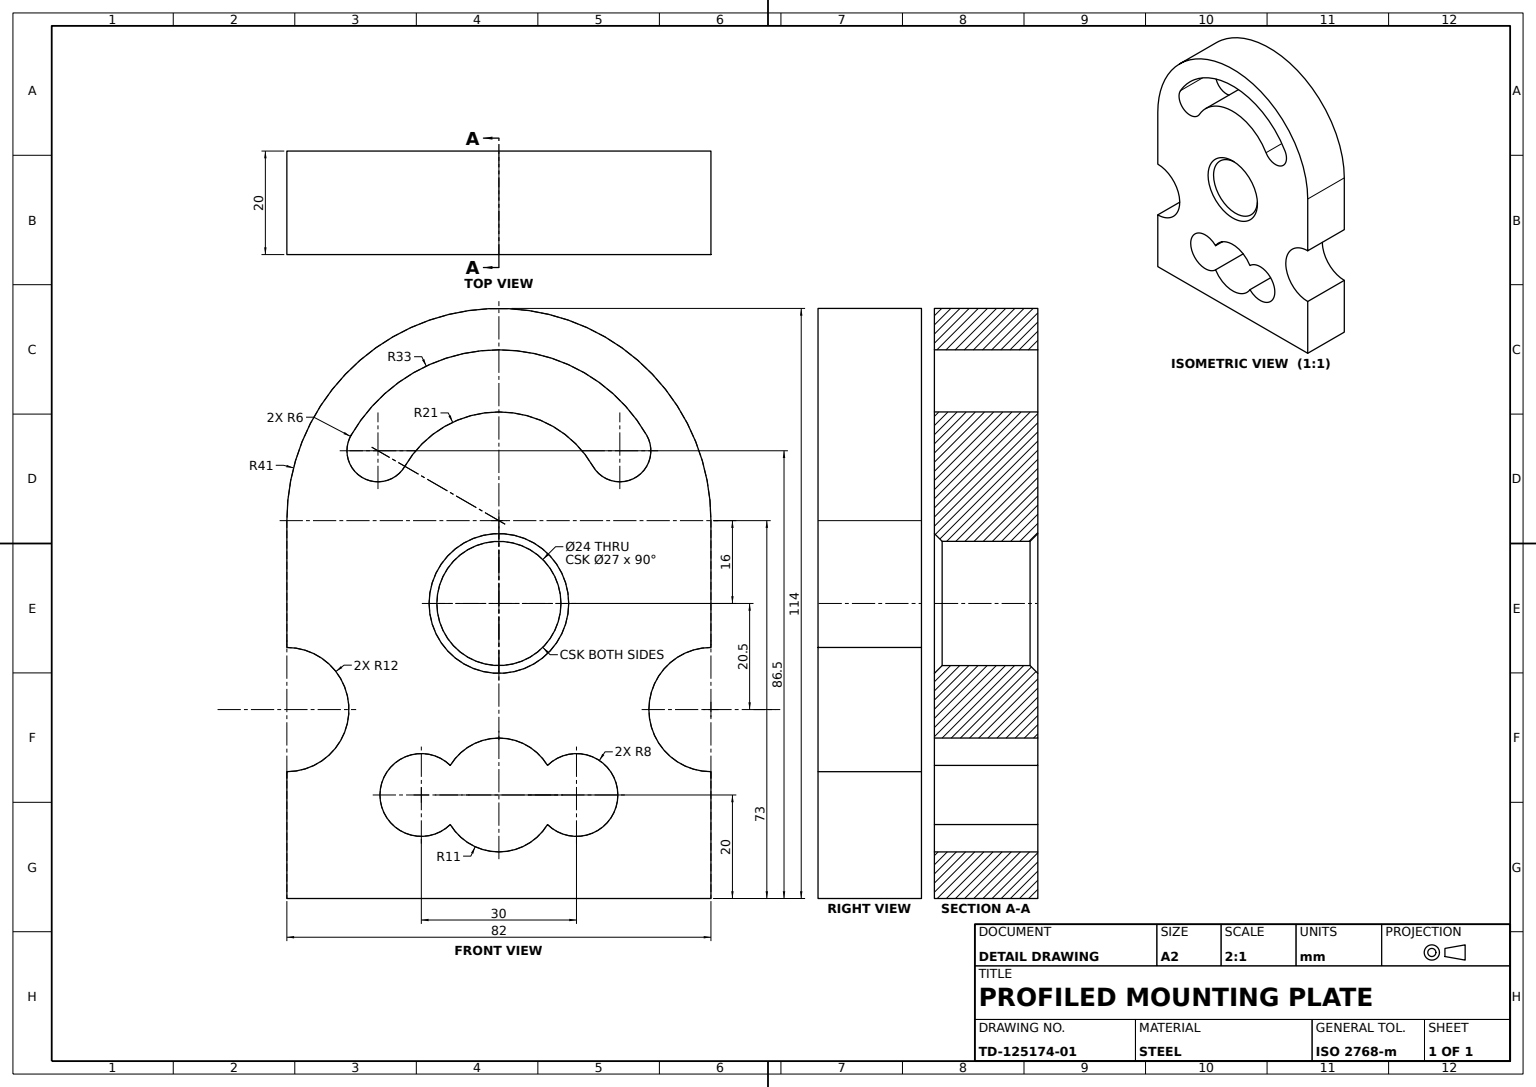
from build123d import *

# Parameters (mm, degrees)
PLATE_PROFILE_SKETCH_R      = 12
PROFILED_PLATE_20MM_DEPTH   = 20
BORE_CHAMFER_1_5X45DEG_SIZE = 1.5


with BuildPart() as part:
    # Plate Profile Sketch → Profiled Plate 20mm (new body)
    with BuildSketch(Plane(origin=(0, 0, 0), x_dir=(0, 0, -1), z_dir=(1, 0, 0))):
        with BuildLine():
            Line((41, 73), (41, 48.5))
            ThreePointArc((41, 48.5), (29, 36.5), (41, 24.5))
            Line((41, 24.5), (41, 0))
            Line((41, 0), (0, 0))
            Line((0, 0), (-41, 0))
            Line((-41, 0), (-41, 24.5))
            ThreePointArc((-41, 24.5), (-29, 36.5), (-41, 48.5))
            Line((-41, 48.5), (-41, 73))
            ThreePointArc((-41, 73), (0, 114), (41, 73))
        make_face()
        with Locations((0, 57)):
            Circle(PLATE_PROFILE_SKETCH_R, mode=Mode.SUBTRACT)
        with BuildLine():
            ThreePointArc((9.4, 25.713142743), (0, 31), (-9.4, 25.713142743))
            ThreePointArc((-9.4, 25.713142743), (-23, 20), (-9.4, 14.286857257))
            ThreePointArc((-9.4, 14.286857257), (0, 9), (9.4, 14.286857257))
            ThreePointArc((9.4, 14.286857257), (23, 20), (9.4, 25.713142743))
        make_face(mode=Mode.SUBTRACT)
        with BuildLine():
            ThreePointArc((28.578838325, 89.5), (0, 106), (-28.578838325, 89.5))
            ThreePointArc((-28.578838325, 89.5), (-26.382685902, 81.303847577), (-18.186533479, 83.5))
            ThreePointArc((-18.186533479, 83.5), (0, 94), (18.186533479, 83.5))
            ThreePointArc((18.186533479, 83.5), (26.382685902, 81.303847577), (28.578838325, 89.5))
        make_face(mode=Mode.SUBTRACT)
    extrude(amount=PROFILED_PLATE_20MM_DEPTH)

    # Bore Chamfer 1.5x45deg
    bore_chamfer_1_5x45deg_edges = [part.edges().sort_by_distance(p)[0] for p in [
        (0, 57, 12),
        (20, 57, 12),
    ]]
    chamfer(bore_chamfer_1_5x45deg_edges, length=BORE_CHAMFER_1_5X45DEG_SIZE)


solid = part.part
